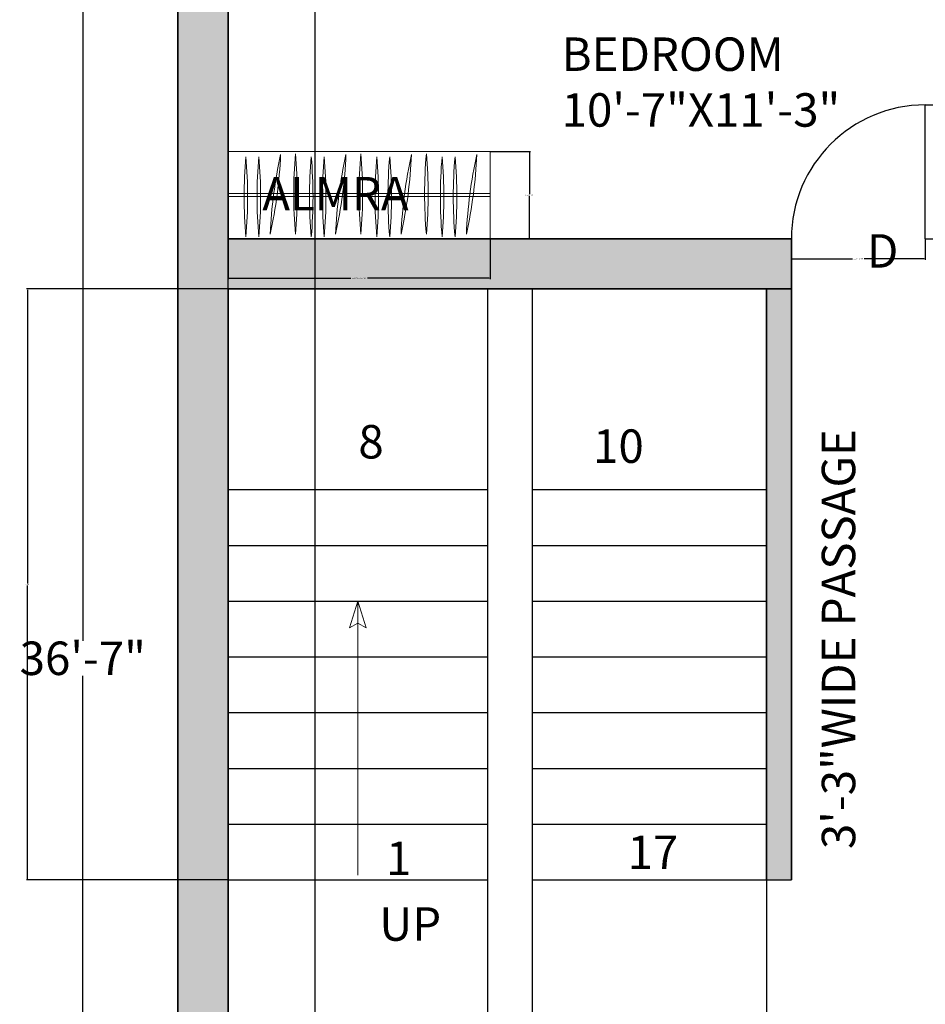
# Model space of a CAD drawing. Units: inches. Extents: x -5 to 330, y -522 to 40.
# Tile 20 of 23: x -5 to 158, y -269 to -92. Entities that reach past the tile are written whole.
import ezdxf

# ---------------------------------------------------------------- set-up
doc = ezdxf.new("R2010")
doc.units = ezdxf.units.IN
doc.header["$MEASUREMENT"] = 0
for name, color, linetype, lineweight in [('A-ANNO-DIMS', 2, 'Continuous', 18), ('A-ANNO-SYMB', 7, 'Continuous', 18), ('A-ANNO-TEXT', 7, 'Continuous', 18), ('A-AREA-IDEN', 7, 'Continuous', 25), ('A-DOOR', 4, 'Continuous', 25), ('A-FLOR-STRS', 7, 'Continuous', 25), ('A-FURN', 8, 'Continuous', 18), ('A-WALL', 7, 'Continuous', 35)]:
    doc.layers.add(name, color=color, linetype=linetype, lineweight=lineweight)
doc.layers.add('A-WALL-PATT', color=18, linetype='Continuous', lineweight=13, true_color=0x000000)
doc.styles.get("Standard").update_dxf_attribs({"font": 'arial.ttf'})
doc.dimstyles.get("Standard").update_dxf_attribs({"dimtxt": 0.18, "dimasz": 0.18, "dimexe": 0.18, "dimexo": 0.0625, "dimgap": 0.09, "dimtad": 0, "dimtih": 1, "dimtoh": 1, "dimdec": 0, "dimzin": 0, "dimdsep": 46, "dimlunit": 3, "dimtxsty": 'Standard', "dimcen": 0.09, "dimadec": 0, "dimazin": 0, "dimtfac": 1, "dimtdec": 0, "dimtofl": 0, "dimtmove": 0, "dimatfit": 3, "dimfxl": 1, "dimtolj": 1, "dimtzin": 0, "dimarcsym": 0})

# ---------------------------------------------------------------- blocks, each defined once
blk = doc.blocks.new('*D2')
at = {"layer": 'A-ANNO-DIMS', "color": 0, "lineweight": -2, "transparency": 16777216}
for p, q in [((23.45, 12.36), (6.27, 12.36)), ((6.45, 12.18), (6.45, -203.74)), ((6.45, -425.96), (6.45, -210.05)), ((23.45, -426.14), (6.27, -426.14))]:
    blk.add_line(p, q, dxfattribs=at)
at = {"layer": 'A-ANNO-DIMS', "color": 0, "transparency": 16777216}
for points in [[(6.42, 12.18), (6.48, 12.18), (6.45, 12.36)], [(6.42, -425.96), (6.48, -425.96), (6.45, -426.14)]]:
    blk.add_solid(points, dxfattribs=at)
at = {"layer": 'Defpoints', "color": 0, "transparency": 16777216}
for p in [(23.51, 12.36), (6.45, -426.14), (23.51, -426.14)]:
    blk.add_point(p, dxfattribs=at)
at = {"layer": 'A-ANNO-DIMS', "color": 0, "transparency": 16777216, "insert": (6.45, -206.89), "char_height": 6, "attachment_point": 5}
blk.add_mtext('\\A1;36\'-7"', dxfattribs=at)
blk = doc.blocks.new('DOOR-24IN-SWING')
blk.add_line((24, 0), (24, 24))
blk.add_arc((24, 0), 24, 90, 180)
blk = doc.blocks.new('WARDROBE-47IN')
for p, q in [((47.01, 15.67), (0, 15.67)), ((0, 15.67), (0, 0)), ((47.01, 15.67), (47.01, 0)), ((47.01, 8.1), (0, 8.1)), ((47.01, 7.57), (0, 7.57)), ((47.01, 0), (0, 0))]:
    blk.add_line(p, q)
for centre, start, end in [((85.32, 7.52), 175.0028, 184.9972), ((-78.95, 7.52), 355.0028, 4.9972), ((87.64, 7.52), 175.0028, 184.9972), ((-76.62, 7.52), 355.0028, 4.9972), ((-72.96, 18.68), 347.508, 357.5023), ((89.91, -2.75), 167.508, 177.5023), ((94.21, 8.03), 175.0028, 184.9972), ((-70.06, 8.03), 355.0028, 4.9972), ((97.03, 7.52), 175.0028, 184.9972), ((-67.23, 7.52), 355.0028, 4.9972), ((99.36, 7.52), 175.0028, 184.9972), ((-64.91, 7.52), 355.0028, 4.9972), ((-61.24, 18.68), 347.508, 357.5023), ((101.62, -2.75), 167.508, 177.5023), ((105.92, 8.03), 175.0028, 184.9972), ((-58.34, 8.03), 355.0028, 4.9972), ((108.79, 7.52), 175.0028, 184.9972), ((-55.48, 7.52), 355.0028, 4.9972), ((111.11, 7.52), 175.0028, 184.9972), ((-53.16, 7.52), 355.0028, 4.9972), ((113.38, -2.75), 167.508, 177.5023), ((-49.49, 18.68), 347.508, 357.5023), ((117.68, 8.03), 175.0028, 184.9972), ((-46.59, 8.03), 355.0028, 4.9972), ((120.5, 7.52), 175.0028, 184.9972), ((-43.77, 7.52), 355.0028, 4.9972), ((122.82, 7.52), 175.0028, 184.9972), ((-41.45, 7.52), 355.0028, 4.9972), ((125.09, -2.75), 167.508, 177.5023), ((-37.78, 18.68), 347.508, 357.5023)]:
    blk.add_arc(centre, 82.45, start, end)
blk = doc.blocks.new('*D17')
at = {"layer": 'A-ANNO-DIMS', "color": 0, "lineweight": -2, "transparency": 16777216}
for p, q in [((133.51, -131.71), (133.51, -135.42)), ((157.51, -131.71), (157.51, -135.42)), ((133.69, -135.24), (144.46, -135.24)), ((157.33, -135.24), (146.56, -135.24))]:
    blk.add_line(p, q, dxfattribs=at)
at = {"layer": 'A-ANNO-DIMS', "color": 0, "transparency": 16777216}
for points in [[(133.69, -135.21), (133.69, -135.27), (133.51, -135.24)], [(157.33, -135.21), (157.33, -135.27), (157.51, -135.24)]]:
    blk.add_solid(points, dxfattribs=at)
at = {"layer": 'Defpoints', "color": 0, "transparency": 16777216}
for p in [(133.51, -131.64), (157.51, -131.64), (157.51, -135.24)]:
    blk.add_point(p, dxfattribs=at)
at = {"layer": 'A-ANNO-DIMS', "color": 0, "transparency": 16777216, "insert": (145.51, -135.24), "char_height": 0.18, "attachment_point": 5}
blk.add_mtext('\\A1;DOOR 2\'-0" TYP.', dxfattribs=at)
blk = doc.blocks.new('*D18')
at = {"layer": 'A-ANNO-DIMS', "color": 0, "lineweight": -2, "transparency": 16777216}
for p, q in [((157.57, -107.64), (161.29, -107.64)), ((161.11, -107.82), (161.11, -119.46)), ((161.11, -131.46), (161.11, -119.83)), ((157.57, -131.64), (161.29, -131.64))]:
    blk.add_line(p, q, dxfattribs=at)
at = {"layer": 'A-ANNO-DIMS', "color": 0, "transparency": 16777216}
for points in [[(161.08, -107.82), (161.14, -107.82), (161.11, -107.64)], [(161.08, -131.46), (161.14, -131.46), (161.11, -131.64)]]:
    blk.add_solid(points, dxfattribs=at)
at = {"layer": 'Defpoints', "color": 0, "transparency": 16777216}
for p in [(157.51, -107.64), (161.11, -107.64), (157.51, -131.64)]:
    blk.add_point(p, dxfattribs=at)
at = {"layer": 'A-ANNO-DIMS', "color": 0, "transparency": 16777216, "insert": (161.11, -119.64), "char_height": 0.18, "attachment_point": 5}
blk.add_mtext('\\A1;2\'-0" TYP.', dxfattribs=at)
blk = doc.blocks.new('*D21')
at = {"layer": 'A-ANNO-DIMS', "color": 0, "lineweight": -2, "transparency": 16777216}
for p, q in [((32.51, -131.71), (32.51, -138.87)), ((79.52, -131.71), (79.52, -138.87)), ((32.69, -138.69), (54.53, -138.69)), ((79.34, -138.69), (57.5, -138.69))]:
    blk.add_line(p, q, dxfattribs=at)
at = {"layer": 'A-ANNO-DIMS', "color": 0, "transparency": 16777216}
for points in [[(32.69, -138.66), (32.69, -138.72), (32.51, -138.69)], [(79.34, -138.66), (79.34, -138.72), (79.52, -138.69)]]:
    blk.add_solid(points, dxfattribs=at)
at = {"layer": 'Defpoints', "color": 0, "transparency": 16777216}
for p in [(32.51, -131.64), (79.52, -131.64), (79.52, -138.69)]:
    blk.add_point(p, dxfattribs=at)
at = {"layer": 'A-ANNO-DIMS', "color": 0, "transparency": 16777216, "insert": (56.01, -138.69), "char_height": 0.18, "attachment_point": 5}
blk.add_mtext('\\A1;WARDROBE 3\'-11" TYP.', dxfattribs=at)
blk = doc.blocks.new('*D22')
at = {"layer": 'A-ANNO-DIMS', "color": 0, "lineweight": -2, "transparency": 16777216}
for p, q in [((79.58, -115.97), (86.75, -115.97)), ((86.57, -116.15), (86.57, -123.63)), ((86.57, -131.46), (86.57, -123.99)), ((79.58, -131.64), (86.75, -131.64))]:
    blk.add_line(p, q, dxfattribs=at)
at = {"layer": 'A-ANNO-DIMS', "color": 0, "transparency": 16777216}
for points in [[(86.54, -116.15), (86.6, -116.15), (86.57, -115.97)], [(86.54, -131.46), (86.6, -131.46), (86.57, -131.64)]]:
    blk.add_solid(points, dxfattribs=at)
at = {"layer": 'Defpoints', "color": 0, "transparency": 16777216}
for p in [(79.52, -115.97), (86.57, -115.97), (79.52, -131.64)]:
    blk.add_point(p, dxfattribs=at)
at = {"layer": 'A-ANNO-DIMS', "color": 0, "transparency": 16777216, "insert": (86.57, -123.81), "char_height": 0.18, "attachment_point": 5}
blk.add_mtext('\\A1;1\'-3 1/2" TYP.', dxfattribs=at)
blk = doc.blocks.new('*D40')
at = {"layer": 'A-ANNO-DIMS', "color": 0, "lineweight": -2, "transparency": 16777216}
for p, q in [((32.51, -246.71), (32.51, -522.31)), ((79.01, -246.71), (79.01, -522.31)), ((32.69, -522.13), (55.15, -522.13)), ((78.83, -522.13), (56.37, -522.13))]:
    blk.add_line(p, q, dxfattribs=at)
at = {"layer": 'A-ANNO-DIMS', "color": 0, "transparency": 16777216}
for points in [[(32.69, -522.1), (32.69, -522.16), (32.51, -522.13)], [(78.83, -522.1), (78.83, -522.16), (79.01, -522.13)]]:
    blk.add_solid(points, dxfattribs=at)
at = {"layer": 'Defpoints', "color": 0, "transparency": 16777216}
for p in [(32.51, -246.64), (79.01, -246.64), (79.01, -522.13)]:
    blk.add_point(p, dxfattribs=at)
at = {"layer": 'A-ANNO-DIMS', "color": 0, "transparency": 16777216, "insert": (55.76, -522.13), "char_height": 0.18, "attachment_point": 5}
blk.add_mtext('\\A1;3\'-10 1/2"', dxfattribs=at)
blk = doc.blocks.new('*D41')
at = {"layer": 'A-ANNO-DIMS', "color": 0, "lineweight": -2, "transparency": 16777216}
for p, q in [((87.01, -246.71), (87.01, -522.31)), ((129.01, -246.71), (129.01, -522.31)), ((87.19, -522.13), (107.68, -522.13)), ((128.83, -522.13), (108.34, -522.13))]:
    blk.add_line(p, q, dxfattribs=at)
at = {"layer": 'A-ANNO-DIMS', "color": 0, "transparency": 16777216}
for points in [[(87.19, -522.1), (87.19, -522.16), (87.01, -522.13)], [(128.83, -522.1), (128.83, -522.16), (129.01, -522.13)]]:
    blk.add_solid(points, dxfattribs=at)
at = {"layer": 'Defpoints', "color": 0, "transparency": 16777216}
for p in [(87.01, -246.64), (129.01, -246.64), (129.01, -522.13)]:
    blk.add_point(p, dxfattribs=at)
at = {"layer": 'A-ANNO-DIMS', "color": 0, "transparency": 16777216, "insert": (108.01, -522.13), "char_height": 0.18, "attachment_point": 5}
blk.add_mtext('\\A1;3\'-6"', dxfattribs=at)
blk = doc.blocks.new('*D42')
at = {"layer": 'A-ANNO-DIMS', "color": 0, "lineweight": -2, "transparency": 16777216}
for p, q in [((32.45, -140.64), (-3.66, -140.64)), ((-3.48, -140.82), (-3.48, -193.46)), ((-3.48, -246.46), (-3.48, -193.83)), ((32.45, -246.64), (-3.66, -246.64))]:
    blk.add_line(p, q, dxfattribs=at)
at = {"layer": 'A-ANNO-DIMS', "color": 0, "transparency": 16777216}
for points in [[(-3.51, -140.82), (-3.45, -140.82), (-3.48, -140.64)], [(-3.51, -246.46), (-3.45, -246.46), (-3.48, -246.64)]]:
    blk.add_solid(points, dxfattribs=at)
at = {"layer": 'Defpoints', "color": 0, "transparency": 16777216}
for p in [(32.51, -140.64), (-3.48, -246.64), (32.51, -246.64)]:
    blk.add_point(p, dxfattribs=at)
at = {"layer": 'A-ANNO-DIMS', "color": 0, "transparency": 16777216, "insert": (-3.48, -193.64), "char_height": 0.18, "attachment_point": 5}
blk.add_mtext('\\A1;8\'-10"', dxfattribs=at)
blk = doc.blocks.new('*D43')
at = {"layer": 'A-ANNO-DIMS', "color": 0, "lineweight": -2, "transparency": 16777216}
for p, q in [((32.51, -297.08), (32.51, 39.52)), ((32.69, 39.34), (39.79, 39.34)), ((47.95, 39.34), (40.85, 39.34)), ((48.13, -297.08), (48.13, 39.52))]:
    blk.add_line(p, q, dxfattribs=at)
at = {"layer": 'A-ANNO-DIMS', "color": 0, "transparency": 16777216}
for points in [[(32.69, 39.37), (32.69, 39.31), (32.51, 39.34)], [(47.95, 39.37), (47.95, 39.31), (48.13, 39.34)]]:
    blk.add_solid(points, dxfattribs=at)
at = {"layer": 'Defpoints', "color": 0, "transparency": 16777216}
for p in [(48.13, 39.34), (32.51, -297.14), (48.13, -297.14)]:
    blk.add_point(p, dxfattribs=at)
at = {"layer": 'A-ANNO-DIMS', "color": 0, "transparency": 16777216, "insert": (40.32, 39.34), "char_height": 0.18, "attachment_point": 5}
blk.add_mtext('\\A1;1\'-3 1/2"', dxfattribs=at)

msp = doc.modelspace()

# ---------------------------------------------------------------- hatches: boundary and pattern name
at = {"layer": 'A-WALL-PATT'}
h = msp.add_hatch(color=256, dxfattribs=at)
h.dxf.hatch_style = 1
h.paths.add_polyline_path([(164.01, -44.15), (159.51, -44.15), (159.51, -153.14), (164.01, -153.14)], flags=17)
h.paths.add_polyline_path([(224.01, -188.14), (272.01, -188.14), (272.01, -218.14), (260.01, -218.14), (260.01, -222.64), (272.01, -222.64), (272.01, -292.64), (159.01, -292.64), (159.01, -297.14), (272.01, -297.14), (272.01, -417.14), (245.51, -417.14), (245.51, -426.14), (272.01, -426.14), (272.01, -495.14), (281.01, -495.14), (281.01, 12.36), (23.51, 12.36), (23.51, -426.14), (62.92, -426.14), (62.92, -417.14), (32.51, -417.14), (32.51, -297.14), (48.13, -297.14), (48.13, -292.64), (32.51, -292.64), (32.51, -140.64), (133.51, -140.64), (133.51, -131.64), (32.51, -131.64), (32.51, 3.36), (159.51, 3.36), (164.01, 3.36), (220.01, 3.36), (224.51, 3.36), (272.01, 3.36), (272.01, -179.14), (159.51, -179.14), (159.51, -188.14), (219.51, -188.14), (219.51, -266.64), (224.01, -266.64), (224.01, -222.64), (236.01, -222.64), (236.01, -218.14), (224.01, -218.14)])
h.paths.add_polyline_path([(133.01, -292.64), (128.51, -292.64), (128.51, -297.14), (128.51, -417.14), (122.92, -417.14), (122.92, -426.14), (133.01, -426.14)], flags=17)
h.paths.add_polyline_path([(185.51, -417.14), (159.01, -417.14), (159.01, -426.14), (185.51, -426.14)], flags=17)
h.paths.add_polyline_path([(133.51, -140.64), (129.01, -140.64), (129.01, -246.64), (133.51, -246.64)], flags=17)
h.paths.add_polyline_path([(246.01, -48.64), (224.51, -48.64), (224.51, -27.63), (220.01, -27.63), (220.01, -48.64), (198.6, -48.64), (198.6, -53.14), (246.01, -53.14)], flags=17)

# ---------------------------------------------------------------- linework, layer by layer
at = {"layer": 'A-ANNO-SYMB'}
for p, q in [((55.76, -196.64), (54.25, -201.45)), ((55.76, -245.78), (55.76, -196.64)), ((55.76, -196.64), (57.27, -201.45)), ((54.25, -201.45), (55.76, -200.59)), ((57.27, -201.45), (55.76, -200.59))]:
    msp.add_line(p, q, dxfattribs=at)
at = {"layer": 'A-FLOR-STRS'}
for p, q in [((79.01, -140.64), (79.01, -246.64)), ((87.01, -140.64), (87.01, -246.64)), ((32.51, -176.64), (79.01, -176.64)), ((87.01, -176.64), (129.01, -176.64)), ((32.51, -186.64), (79.01, -186.64)), ((87.01, -186.64), (129.01, -186.64)), ((32.51, -196.64), (79.01, -196.64)), ((87.01, -196.64), (129.01, -196.64)), ((32.51, -206.64), (79.01, -206.64)), ((87.01, -206.64), (129.01, -206.64)), ((32.51, -216.64), (79.01, -216.64)), ((87.01, -216.64), (129.01, -216.64)), ((32.51, -226.64), (79.01, -226.64)), ((87.01, -226.64), (129.01, -226.64)), ((32.51, -236.64), (79.01, -236.64)), ((87.01, -236.64), (129.01, -236.64)), ((32.51, -246.64), (79.01, -246.64)), ((87.01, -246.64), (133.51, -246.64))]:
    msp.add_line(p, q, dxfattribs=at)
at = {"layer": 'A-WALL'}
for p, q in [((23.51, 12.36), (23.51, -495.14)), ((32.51, 3.36), (32.51, -131.64)), ((32.51, -131.64), (133.51, -131.64)), ((133.51, -140.64), (133.51, -131.64)), ((32.51, -140.64), (133.51, -140.64)), ((32.51, -140.64), (32.51, -292.64)), ((129.01, -140.64), (129.01, -246.64)), ((133.51, -140.64), (133.51, -246.64))]:
    msp.add_line(p, q, dxfattribs=at)

# ---------------------------------------------------------------- block references
at = {"layer": 'A-DOOR'}
msp.add_blockref('DOOR-24IN-SWING', (133.51, -131.64), dxfattribs=at)
at = {"layer": 'A-FURN'}
msp.add_blockref('WARDROBE-47IN', (32.51, -131.64), dxfattribs=at)

# ---------------------------------------------------------------- texts
at = {"layer": 'A-ANNO-TEXT', "insert": (38.64, -120.57), "char_height": 6, "attachment_point": 1}
msp.add_mtext_dynamic_manual_height_columns('ALMRA', width=37.1962, gutter_width=1, heights=[0], dxfattribs=at)
at = {"layer": 'A-ANNO-TEXT', "char_height": 6, "attachment_point": 1}
for s, insert in [('D', (147.05, -130.83)), ('8', (55.86, -165.05)), ('10', (97.95, -165.84)), ('1', (60.84, -239.76)), ('17', (104.14, -238.68)), ('UP', (59.62, -251.55))]:
    msp.add_mtext(s, dxfattribs=dict(at, insert=insert))
at = {"layer": 'A-AREA-IDEN', "insert": (92.31, -95.54), "char_height": 6, "attachment_point": 1}
msp.add_mtext('BEDROOM\\P10\'-7"X11\'-3"', dxfattribs=at)
at = {"layer": 'A-AREA-IDEN', "insert": (138.95, -241.11), "char_height": 6, "attachment_point": 1, "rotation": 90}
msp.add_mtext('3\'-3"WIDE PASSAGE', dxfattribs=at)

# ---------------------------------------------------------------- dimensions: what is measured, and where the dimension line sits
at = {"layer": 'A-ANNO-DIMS'}
for base, p1, p2, picture, middle in [((48.13, 39.34), (32.51, -297.14), (48.13, -297.14), '*D43', (40.32, 39.34)), ((79.01, -522.13), (32.51, -246.64), (79.01, -246.64), '*D40', (55.76, -522.13)), ((129.01, -522.13), (87.01, -246.64), (129.01, -246.64), '*D41', (108.01, -522.13))]:
    dim = msp.add_linear_dim(base=base, p1=p1, p2=p2, dimstyle='Standard', override={"dimdec": 1, "dimlfac": 1, "dimrnd": 0, "dimzin": 1, "dimdsep": 46, "dimlunit": 4, "dimfrac": 2}, dxfattribs=at)
    dim.commit()
    dim.dimension.update_dxf_attribs({"geometry": picture, "text_midpoint": middle})
for base, p1, p2, override, picture, middle in [((6.45432189, -426.14358203), (23.50988858, 12.35641797), (23.50988858, -426.14358203), {"dimtxt": 6, "dimclrd": 0, "dimclre": 0, "dimclrt": 0}, '*D2', (6.45432189, -206.89358203)), ((-3.48, -246.64), (32.51, -140.64), (32.51, -246.64), {"dimdec": 1, "dimlfac": 1, "dimrnd": 0, "dimzin": 1, "dimdsep": 46, "dimlunit": 4, "dimfrac": 2}, '*D42', (-3.48, -193.64))]:
    dim = msp.add_linear_dim(base=base, p1=p1, p2=p2, angle=90, dimstyle='Standard', override=override, dxfattribs=at)
    dim.commit()
    dim.dimension.update_dxf_attribs({"geometry": picture, "text_midpoint": middle})
for base, p1, p2, picture, middle in [((161.11, -107.64), (157.51, -131.64), (157.51, -107.64), '*D18', (161.11, -119.64)), ((86.57, -115.97), (79.52, -131.64), (79.52, -115.97), '*D22', (86.57, -123.81))]:
    dim = msp.add_linear_dim(base=base, p1=p1, p2=p2, angle=90, text='<> TYP.', dimstyle='Standard', override={"dimdec": 1, "dimlfac": 1, "dimrnd": 0, "dimzin": 1, "dimdsep": 46, "dimlunit": 4, "dimfrac": 2}, dxfattribs=at)
    dim.commit()
    dim.dimension.update_dxf_attribs({"geometry": picture, "text_midpoint": middle})
for base, p1, p2, text, picture, middle in [((79.52, -138.69), (32.51, -131.64), (79.52, -131.64), 'WARDROBE <> TYP.', '*D21', (56.01, -138.69)), ((157.51, -135.24), (133.51, -131.64), (157.51, -131.64), 'DOOR <> TYP.', '*D17', (145.51, -135.24))]:
    dim = msp.add_linear_dim(base=base, p1=p1, p2=p2, text=text, dimstyle='Standard', override={"dimdec": 1, "dimlfac": 1, "dimrnd": 0, "dimzin": 1, "dimdsep": 46, "dimlunit": 4, "dimfrac": 2}, dxfattribs=at)
    dim.commit()
    dim.dimension.update_dxf_attribs({"geometry": picture, "text_midpoint": middle})

doc.saveas('drawing.dxf')
